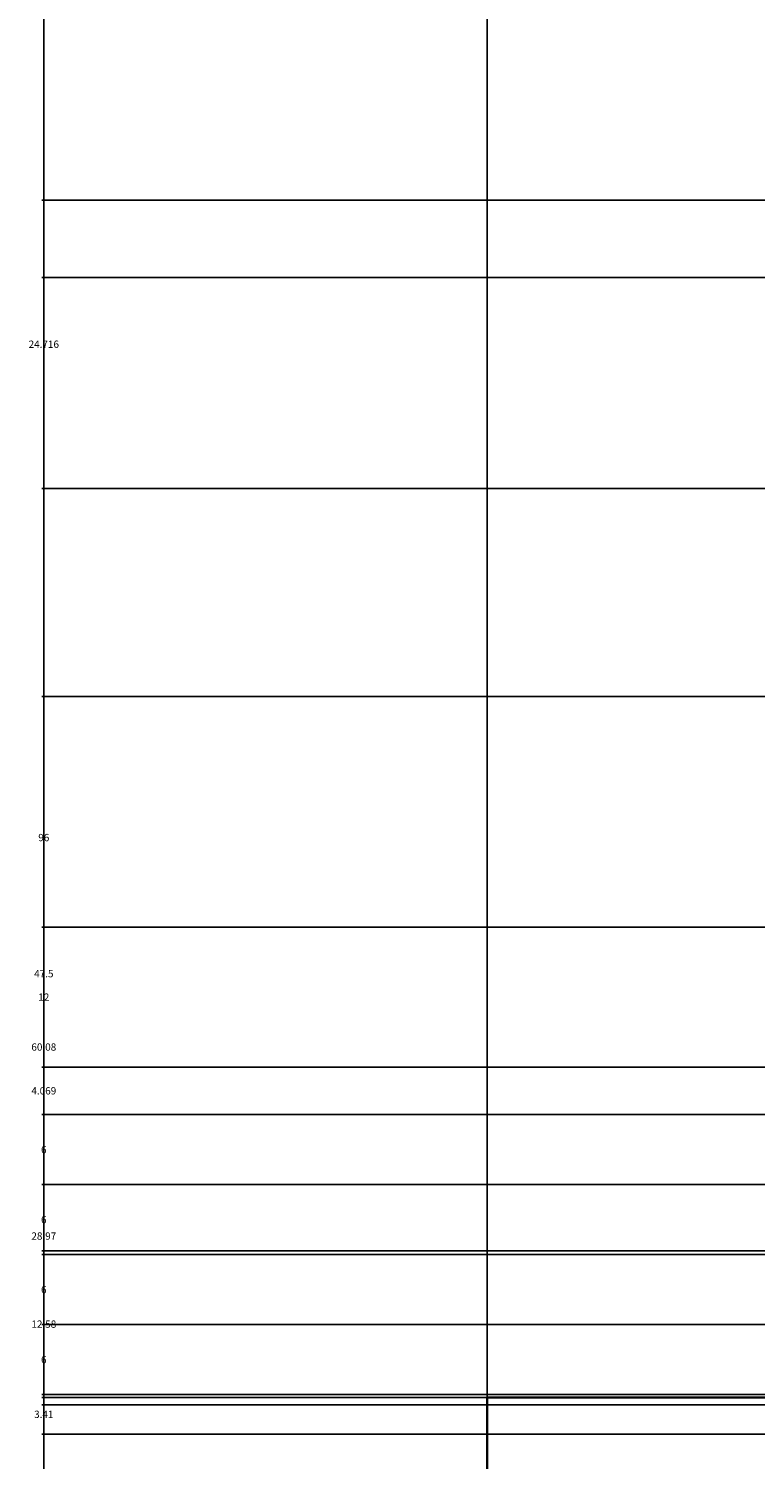
# Model space of a CAD drawing. Units: inches. Extents: x -13 to 809, y 112 to 656.
# Tile 3 of 55: x -13 to 49, y 205 to 328. Entities that reach past the tile are written whole.
import ezdxf

# ---------------------------------------------------------------- set-up
doc = ezdxf.new("R2010")
doc.units = ezdxf.units.IN
doc.header["$MEASUREMENT"] = 0
doc.layers.add('A-ANNO-DIMS', color=2, linetype='Continuous', lineweight=18)
doc.layers.add('A-ELEV', color=7, linetype='Continuous', lineweight=35)
doc.styles.get("Standard").update_dxf_attribs({"font": 'arial.ttf'})
doc.dimstyles.get("Standard").update_dxf_attribs({"dimtxt": 0.625, "dimasz": 0.18, "dimexe": 0.18, "dimexo": 0.0625, "dimgap": 0.09, "dimtad": 0, "dimtih": 1, "dimtoh": 1, "dimdec": 4, "dimzin": 0, "dimdsep": 46, "dimlunit": 4, "dimtxsty": 'Standard', "dimcen": 0.09, "dimadec": 0, "dimazin": 0, "dimtfac": 1, "dimtdec": 4, "dimtofl": 0, "dimtmove": 0, "dimatfit": 3, "dimfxl": 1, "dimtolj": 1, "dimtzin": 0, "dimarcsym": 0})

# ---------------------------------------------------------------- blocks, each defined once
blk = doc.blocks.new('*D11')
at = {"layer": 'A-ANNO-DIMS', "color": 0, "lineweight": -2, "transparency": 16777216}
for p, q in [((95.05, 306.46), (95.05, 112.34)), ((26.08, 150.46), (26.08, 112.34)), ((26.26, 112.52), (59.42, 112.52)), ((94.87, 112.52), (61.71, 112.52))]:
    blk.add_line(p, q, dxfattribs=at)
at = {"layer": 'A-ANNO-DIMS', "color": 0, "transparency": 16777216}
for points in [[(26.26, 112.55), (26.26, 112.49), (26.08, 112.52)], [(94.87, 112.55), (94.87, 112.49), (95.05, 112.52)]]:
    blk.add_solid(points, dxfattribs=at)
at = {"layer": 'Defpoints', "color": 0, "transparency": 16777216}
for p in [(95.05, 306.52), (26.08, 150.52), (95.05, 112.52)]:
    blk.add_point(p, dxfattribs=at)
at = {"layer": 'A-ANNO-DIMS', "color": 0, "transparency": 16777216, "insert": (60.56, 112.52), "char_height": 0.625, "attachment_point": 5}
blk.add_mtext('\\A1;68.97', dxfattribs=at)
blk = doc.blocks.new('*D22')
at = {"layer": 'A-ANNO-DIMS', "color": 0, "lineweight": -2, "transparency": 16777216}
for p, q in [((26.08, 210.58), (26.08, 655.96)), ((26.26, 655.78), (65.52, 655.78)), ((107.08, 655.78), (67.82, 655.78)), ((107.26, 510.58), (107.26, 655.96))]:
    blk.add_line(p, q, dxfattribs=at)
at = {"layer": 'A-ANNO-DIMS', "color": 0, "transparency": 16777216}
for points in [[(26.26, 655.81), (26.26, 655.75), (26.08, 655.78)], [(107.08, 655.81), (107.08, 655.75), (107.26, 655.78)]]:
    blk.add_solid(points, dxfattribs=at)
at = {"layer": 'Defpoints', "color": 0, "transparency": 16777216}
for p in [(107.26, 655.78), (107.26, 510.52), (26.08, 210.52)]:
    blk.add_point(p, dxfattribs=at)
at = {"layer": 'A-ANNO-DIMS', "color": 0, "transparency": 16777216, "insert": (66.67, 655.78), "char_height": 0.625, "attachment_point": 5}
blk.add_mtext('\\A1;81.18', dxfattribs=at)
blk = doc.blocks.new('*D32')
at = {"layer": 'A-ANNO-DIMS', "color": 0, "lineweight": -2, "transparency": 16777216}
for p, q in [((26.02, 210.52), (-12.1, 210.52)), ((-11.92, 210.34), (-11.92, 180.93)), ((-11.92, 150.7), (-11.92, 180.11)), ((26.02, 150.52), (-12.1, 150.52))]:
    blk.add_line(p, q, dxfattribs=at)
at = {"layer": 'A-ANNO-DIMS', "color": 0, "transparency": 16777216}
for points in [[(-11.95, 210.34), (-11.89, 210.34), (-11.92, 210.52)], [(-11.95, 150.7), (-11.89, 150.7), (-11.92, 150.52)]]:
    blk.add_solid(points, dxfattribs=at)
at = {"layer": 'Defpoints', "color": 0, "transparency": 16777216}
for p in [(-11.92, 210.52), (26.08, 210.52), (26.08, 150.52)]:
    blk.add_point(p, dxfattribs=at)
at = {"layer": 'A-ANNO-DIMS', "color": 0, "transparency": 16777216, "insert": (-11.92, 180.52), "char_height": 0.625, "attachment_point": 5}
blk.add_mtext('\\A1;60', dxfattribs=at)
blk = doc.blocks.new('*D33')
at = {"layer": 'A-ANNO-DIMS', "color": 0, "lineweight": -2, "transparency": 16777216}
for p, q in [((94.98, 306.52), (-12.1, 306.52)), ((-11.92, 306.34), (-11.92, 258.93)), ((-11.92, 210.7), (-11.92, 258.11)), ((26.02, 210.52), (-12.1, 210.52))]:
    blk.add_line(p, q, dxfattribs=at)
at = {"layer": 'A-ANNO-DIMS', "color": 0, "transparency": 16777216}
for points in [[(-11.95, 306.34), (-11.89, 306.34), (-11.92, 306.52)], [(-11.95, 210.7), (-11.89, 210.7), (-11.92, 210.52)]]:
    blk.add_solid(points, dxfattribs=at)
at = {"layer": 'Defpoints', "color": 0, "transparency": 16777216}
for p in [(-11.92, 306.52), (95.05, 306.52), (26.08, 210.52)]:
    blk.add_point(p, dxfattribs=at)
at = {"layer": 'A-ANNO-DIMS', "color": 0, "transparency": 16777216, "insert": (-11.92, 258.52), "char_height": 0.625, "attachment_point": 5}
blk.add_mtext('\\A1;96', dxfattribs=at)
blk = doc.blocks.new('*D34')
at = {"layer": 'A-ANNO-DIMS', "color": 0, "lineweight": -2, "transparency": 16777216}
for p, q in [((94.98, 462.52), (-12.1, 462.52)), ((-11.92, 462.34), (-11.92, 384.93)), ((-11.92, 306.7), (-11.92, 384.11)), ((94.98, 306.52), (-12.1, 306.52))]:
    blk.add_line(p, q, dxfattribs=at)
at = {"layer": 'A-ANNO-DIMS', "color": 0, "transparency": 16777216}
for points in [[(-11.95, 462.34), (-11.89, 462.34), (-11.92, 462.52)], [(-11.95, 306.7), (-11.89, 306.7), (-11.92, 306.52)]]:
    blk.add_solid(points, dxfattribs=at)
at = {"layer": 'Defpoints', "color": 0, "transparency": 16777216}
for p in [(-11.92, 462.52), (95.05, 462.52), (95.05, 306.52)]:
    blk.add_point(p, dxfattribs=at)
at = {"layer": 'A-ANNO-DIMS', "color": 0, "transparency": 16777216, "insert": (-11.92, 384.52), "char_height": 0.625, "attachment_point": 5}
blk.add_mtext('\\A1;156', dxfattribs=at)
blk = doc.blocks.new('*D39')
at = {"layer": 'A-ANNO-DIMS', "color": 0, "lineweight": -2, "transparency": 16777216}
for p, q in [((341.34, 524.28), (-12.1, 524.28)), ((-11.92, 524.1), (-11.92, 406.78)), ((-11.92, 288.63), (-11.92, 405.96)), ((341.34, 288.45), (-12.1, 288.45))]:
    blk.add_line(p, q, dxfattribs=at)
at = {"layer": 'A-ANNO-DIMS', "color": 0, "transparency": 16777216}
for points in [[(-11.95, 524.1), (-11.89, 524.1), (-11.92, 524.28)], [(-11.95, 288.63), (-11.89, 288.63), (-11.92, 288.45)]]:
    blk.add_solid(points, dxfattribs=at)
at = {"layer": 'Defpoints', "color": 0, "transparency": 16777216}
for p in [(-11.92, 524.28), (341.41, 524.28), (341.41, 288.45)]:
    blk.add_point(p, dxfattribs=at)
at = {"layer": 'A-ANNO-DIMS', "color": 0, "transparency": 16777216, "insert": (-11.92, 406.37), "char_height": 0.625, "attachment_point": 5}
blk.add_mtext('\\A1;235.83', dxfattribs=at)
blk = doc.blocks.new('*D40')
at = {"layer": 'A-ANNO-DIMS', "color": 0, "lineweight": -2, "transparency": 16777216}
for p, q in [((471.04, 313.17), (-12.1, 313.17)), ((-11.92, 312.99), (-11.92, 301.22)), ((-11.92, 288.63), (-11.92, 300.4)), ((341.34, 288.45), (-12.1, 288.45))]:
    blk.add_line(p, q, dxfattribs=at)
at = {"layer": 'A-ANNO-DIMS', "color": 0, "transparency": 16777216}
for points in [[(-11.95, 312.99), (-11.89, 312.99), (-11.92, 313.17)], [(-11.95, 288.63), (-11.89, 288.63), (-11.92, 288.45)]]:
    blk.add_solid(points, dxfattribs=at)
at = {"layer": 'Defpoints', "color": 0, "transparency": 16777216}
for p in [(471.1, 313.17), (-11.92, 288.45), (341.41, 288.45)]:
    blk.add_point(p, dxfattribs=at)
at = {"layer": 'A-ANNO-DIMS', "color": 0, "transparency": 16777216, "insert": (-11.92, 300.81), "char_height": 0.625, "attachment_point": 5}
blk.add_mtext('\\A1;24.716', dxfattribs=at)
blk = doc.blocks.new('*D41')
at = {"layer": 'A-ANNO-DIMS', "color": 0, "lineweight": -2, "transparency": 16777216}
for p, q in [((471.04, 357.98), (-12.1, 357.98)), ((-11.92, 357.8), (-11.92, 335.98)), ((-11.92, 313.35), (-11.92, 335.16)), ((471.04, 313.17), (-12.1, 313.17))]:
    blk.add_line(p, q, dxfattribs=at)
at = {"layer": 'A-ANNO-DIMS', "color": 0, "transparency": 16777216}
for points in [[(-11.95, 357.8), (-11.89, 357.8), (-11.92, 357.98)], [(-11.95, 313.35), (-11.89, 313.35), (-11.92, 313.17)]]:
    blk.add_solid(points, dxfattribs=at)
at = {"layer": 'Defpoints', "color": 0, "transparency": 16777216}
for p in [(-11.92, 357.98), (471.1, 357.98), (471.1, 313.17)]:
    blk.add_point(p, dxfattribs=at)
at = {"layer": 'A-ANNO-DIMS', "color": 0, "transparency": 16777216, "insert": (-11.92, 335.57), "char_height": 0.625, "attachment_point": 5}
blk.add_mtext('\\A1;44.81', dxfattribs=at)
blk = doc.blocks.new('*D44')
at = {"layer": 'A-ANNO-DIMS', "color": 0, "lineweight": -2, "transparency": 16777216}
for p, q in [((124.86, 270.6), (-12.1, 270.6)), ((-11.92, 270.42), (-11.92, 240.97)), ((-11.92, 210.7), (-11.92, 240.15)), ((124.86, 210.52), (-12.1, 210.52))]:
    blk.add_line(p, q, dxfattribs=at)
at = {"layer": 'A-ANNO-DIMS', "color": 0, "transparency": 16777216}
for points in [[(-11.95, 270.42), (-11.89, 270.42), (-11.92, 270.6)], [(-11.95, 210.7), (-11.89, 210.7), (-11.92, 210.52)]]:
    blk.add_solid(points, dxfattribs=at)
at = {"layer": 'Defpoints', "color": 0, "transparency": 16777216}
for p in [(-11.92, 270.6), (124.92, 270.6), (124.92, 210.52)]:
    blk.add_point(p, dxfattribs=at)
at = {"layer": 'A-ANNO-DIMS', "color": 0, "transparency": 16777216, "insert": (-11.92, 240.56), "char_height": 0.625, "attachment_point": 5}
blk.add_mtext('\\A1;60.08', dxfattribs=at)
blk = doc.blocks.new('*D45')
at = {"layer": 'A-ANNO-DIMS', "color": 0, "lineweight": -2, "transparency": 16777216}
for p, q in [((275.65, 270.6), (-12.1, 270.6)), ((-11.92, 270.42), (-11.92, 247.26)), ((-11.92, 223.28), (-11.92, 246.44)), ((275.65, 223.1), (-12.1, 223.1))]:
    blk.add_line(p, q, dxfattribs=at)
at = {"layer": 'A-ANNO-DIMS', "color": 0, "transparency": 16777216}
for points in [[(-11.95, 270.42), (-11.89, 270.42), (-11.92, 270.6)], [(-11.95, 223.28), (-11.89, 223.28), (-11.92, 223.1)]]:
    blk.add_solid(points, dxfattribs=at)
at = {"layer": 'Defpoints', "color": 0, "transparency": 16777216}
for p in [(-11.92, 270.6), (275.71, 270.6), (275.71, 223.1)]:
    blk.add_point(p, dxfattribs=at)
at = {"layer": 'A-ANNO-DIMS', "color": 0, "transparency": 16777216, "insert": (-11.92, 246.85), "char_height": 0.625, "attachment_point": 5}
blk.add_mtext('\\A1;47.5', dxfattribs=at)
blk = doc.blocks.new('*D49')
at = {"layer": 'A-ANNO-DIMS', "color": 0, "lineweight": -2, "transparency": 16777216}
for p, q in [((590.95, 250.84), (-12.1, 250.84)), ((-11.92, 250.66), (-11.92, 245.25)), ((-11.92, 239.02), (-11.92, 244.44)), ((590.95, 238.84), (-12.1, 238.84))]:
    blk.add_line(p, q, dxfattribs=at)
at = {"layer": 'A-ANNO-DIMS', "color": 0, "transparency": 16777216}
for points in [[(-11.95, 250.66), (-11.89, 250.66), (-11.92, 250.84)], [(-11.95, 239.02), (-11.89, 239.02), (-11.92, 238.84)]]:
    blk.add_solid(points, dxfattribs=at)
at = {"layer": 'Defpoints', "color": 0, "transparency": 16777216}
for p in [(-11.92, 250.84), (591.01, 250.84), (591.01, 238.84)]:
    blk.add_point(p, dxfattribs=at)
at = {"layer": 'A-ANNO-DIMS', "color": 0, "transparency": 16777216, "insert": (-11.92, 244.84), "char_height": 0.625, "attachment_point": 5}
blk.add_mtext('\\A1;12', dxfattribs=at)
blk = doc.blocks.new('*D50')
at = {"layer": 'A-ANNO-DIMS', "color": 0, "lineweight": -2, "transparency": 16777216}
for p, q in [((590.95, 238.84), (-12.1, 238.84)), ((-11.92, 238.66), (-11.92, 224.77)), ((-11.92, 210.06), (-11.92, 223.95)), ((607.51, 209.88), (-12.1, 209.88))]:
    blk.add_line(p, q, dxfattribs=at)
at = {"layer": 'A-ANNO-DIMS', "color": 0, "transparency": 16777216}
for points in [[(-11.95, 238.66), (-11.89, 238.66), (-11.92, 238.84)], [(-11.95, 210.06), (-11.89, 210.06), (-11.92, 209.88)]]:
    blk.add_solid(points, dxfattribs=at)
at = {"layer": 'Defpoints', "color": 0, "transparency": 16777216}
for p in [(591.01, 238.84), (-11.92, 209.88), (607.57, 209.88)]:
    blk.add_point(p, dxfattribs=at)
at = {"layer": 'A-ANNO-DIMS', "color": 0, "transparency": 16777216, "insert": (-11.92, 224.36), "char_height": 0.625, "attachment_point": 5}
blk.add_mtext('\\A1;28.97', dxfattribs=at)
blk = doc.blocks.new('*D80')
at = {"layer": 'A-ANNO-DIMS', "color": 0, "lineweight": -2, "transparency": 16777216}
for p, q in [((368.83, 216.77), (-12.1, 216.77)), ((-11.92, 216.59), (-11.92, 214.18)), ((-11.92, 210.95), (-11.92, 213.36)), ((368.83, 210.77), (-12.1, 210.77))]:
    blk.add_line(p, q, dxfattribs=at)
at = {"layer": 'A-ANNO-DIMS', "color": 0, "transparency": 16777216}
for points in [[(-11.95, 216.59), (-11.89, 216.59), (-11.92, 216.77)], [(-11.95, 210.95), (-11.89, 210.95), (-11.92, 210.77)]]:
    blk.add_solid(points, dxfattribs=at)
at = {"layer": 'Defpoints', "color": 0, "transparency": 16777216}
for p in [(-11.92, 216.77), (368.9, 216.77), (368.9, 210.77)]:
    blk.add_point(p, dxfattribs=at)
at = {"layer": 'A-ANNO-DIMS', "color": 0, "transparency": 16777216, "insert": (-11.92, 213.77), "char_height": 0.625, "attachment_point": 5}
blk.add_mtext('\\A1;6', dxfattribs=at)
blk = doc.blocks.new('*D81')
at = {"layer": 'A-ANNO-DIMS', "color": 0, "lineweight": -2, "transparency": 16777216}
for p, q in [((378.83, 222.77), (-12.1, 222.77)), ((-11.92, 222.59), (-11.92, 220.18)), ((-11.92, 216.95), (-11.92, 219.36)), ((378.83, 216.77), (-12.1, 216.77))]:
    blk.add_line(p, q, dxfattribs=at)
at = {"layer": 'A-ANNO-DIMS', "color": 0, "transparency": 16777216}
for points in [[(-11.95, 222.59), (-11.89, 222.59), (-11.92, 222.77)], [(-11.95, 216.95), (-11.89, 216.95), (-11.92, 216.77)]]:
    blk.add_solid(points, dxfattribs=at)
at = {"layer": 'Defpoints', "color": 0, "transparency": 16777216}
for p in [(-11.92, 222.77), (378.9, 222.77), (378.9, 216.77)]:
    blk.add_point(p, dxfattribs=at)
at = {"layer": 'A-ANNO-DIMS', "color": 0, "transparency": 16777216, "insert": (-11.92, 219.77), "char_height": 0.625, "attachment_point": 5}
blk.add_mtext('\\A1;6', dxfattribs=at)
blk = doc.blocks.new('*D82')
at = {"layer": 'A-ANNO-DIMS', "color": 0, "lineweight": -2, "transparency": 16777216}
for p, q in [((388.83, 228.77), (-12.1, 228.77)), ((-11.92, 228.59), (-11.92, 226.18)), ((-11.92, 222.95), (-11.92, 225.36)), ((388.83, 222.77), (-12.1, 222.77))]:
    blk.add_line(p, q, dxfattribs=at)
at = {"layer": 'A-ANNO-DIMS', "color": 0, "transparency": 16777216}
for points in [[(-11.95, 228.59), (-11.89, 228.59), (-11.92, 228.77)], [(-11.95, 222.95), (-11.89, 222.95), (-11.92, 222.77)]]:
    blk.add_solid(points, dxfattribs=at)
at = {"layer": 'Defpoints', "color": 0, "transparency": 16777216}
for p in [(-11.92, 228.77), (388.9, 228.77), (388.9, 222.77)]:
    blk.add_point(p, dxfattribs=at)
at = {"layer": 'A-ANNO-DIMS', "color": 0, "transparency": 16777216, "insert": (-11.92, 225.77), "char_height": 0.625, "attachment_point": 5}
blk.add_mtext('\\A1;6', dxfattribs=at)
blk = doc.blocks.new('*D83')
at = {"layer": 'A-ANNO-DIMS', "color": 0, "lineweight": -2, "transparency": 16777216}
for p, q in [((398.83, 234.77), (-12.1, 234.77)), ((-11.92, 234.59), (-11.92, 232.18)), ((-11.92, 228.95), (-11.92, 231.36)), ((398.83, 228.77), (-12.1, 228.77))]:
    blk.add_line(p, q, dxfattribs=at)
at = {"layer": 'A-ANNO-DIMS', "color": 0, "transparency": 16777216}
for points in [[(-11.95, 234.59), (-11.89, 234.59), (-11.92, 234.77)], [(-11.95, 228.95), (-11.89, 228.95), (-11.92, 228.77)]]:
    blk.add_solid(points, dxfattribs=at)
at = {"layer": 'Defpoints', "color": 0, "transparency": 16777216}
for p in [(-11.92, 234.77), (398.9, 234.77), (398.9, 228.77)]:
    blk.add_point(p, dxfattribs=at)
at = {"layer": 'A-ANNO-DIMS', "color": 0, "transparency": 16777216, "insert": (-11.92, 231.77), "char_height": 0.625, "attachment_point": 5}
blk.add_mtext('\\A1;6', dxfattribs=at)
blk = doc.blocks.new('*D84')
at = {"layer": 'A-ANNO-DIMS', "color": 0, "lineweight": -2, "transparency": 16777216}
for p, q in [((408.83, 238.84), (-12.1, 238.84)), ((-11.92, 238.66), (-11.92, 237.22)), ((-11.92, 234.95), (-11.92, 236.4)), ((408.83, 234.77), (-12.1, 234.77))]:
    blk.add_line(p, q, dxfattribs=at)
at = {"layer": 'A-ANNO-DIMS', "color": 0, "transparency": 16777216}
for points in [[(-11.95, 238.66), (-11.89, 238.66), (-11.92, 238.84)], [(-11.95, 234.95), (-11.89, 234.95), (-11.92, 234.77)]]:
    blk.add_solid(points, dxfattribs=at)
at = {"layer": 'Defpoints', "color": 0, "transparency": 16777216}
for p in [(-11.92, 238.84), (408.9, 238.84), (408.9, 234.77)]:
    blk.add_point(p, dxfattribs=at)
at = {"layer": 'A-ANNO-DIMS', "color": 0, "transparency": 16777216, "insert": (-11.92, 236.81), "char_height": 0.625, "attachment_point": 5}
blk.add_mtext('\\A1;4.069', dxfattribs=at)
blk = doc.blocks.new('*D90')
at = {"layer": 'A-ANNO-DIMS', "color": 0, "lineweight": -2, "transparency": 16777216}
for p, q in [((26.08, 210.46), (26.08, 112.34)), ((76.47, 195.83), (76.47, 112.34)), ((26.26, 112.52), (50.13, 112.52)), ((76.29, 112.52), (52.42, 112.52))]:
    blk.add_line(p, q, dxfattribs=at)
at = {"layer": 'A-ANNO-DIMS', "color": 0, "transparency": 16777216}
for points in [[(26.26, 112.55), (26.26, 112.49), (26.08, 112.52)], [(76.29, 112.55), (76.29, 112.49), (76.47, 112.52)]]:
    blk.add_solid(points, dxfattribs=at)
at = {"layer": 'Defpoints', "color": 0, "transparency": 16777216}
for p in [(26.08, 210.52), (76.47, 195.89), (76.47, 112.52)]:
    blk.add_point(p, dxfattribs=at)
at = {"layer": 'A-ANNO-DIMS', "color": 0, "transparency": 16777216, "insert": (51.28, 112.52), "char_height": 0.625, "attachment_point": 5}
blk.add_mtext('\\A1;50.39', dxfattribs=at)
blk = doc.blocks.new('*D94')
at = {"layer": 'A-ANNO-DIMS', "color": 0, "lineweight": -2, "transparency": 16777216}
for p, q in [((210.02, 223.1), (-12.1, 223.1)), ((-11.92, 222.92), (-11.92, 217.22)), ((-11.92, 210.7), (-11.92, 216.4)), ((160.86, 210.52), (-12.1, 210.52))]:
    blk.add_line(p, q, dxfattribs=at)
at = {"layer": 'A-ANNO-DIMS', "color": 0, "transparency": 16777216}
for points in [[(-11.95, 222.92), (-11.89, 222.92), (-11.92, 223.1)], [(-11.95, 210.7), (-11.89, 210.7), (-11.92, 210.52)]]:
    blk.add_solid(points, dxfattribs=at)
at = {"layer": 'Defpoints', "color": 0, "transparency": 16777216}
for p in [(-11.92, 223.1), (210.08, 223.1), (160.92, 210.52)]:
    blk.add_point(p, dxfattribs=at)
at = {"layer": 'A-ANNO-DIMS', "color": 0, "transparency": 16777216, "insert": (-11.92, 216.81), "char_height": 0.625, "attachment_point": 5}
blk.add_mtext('\\A1;12.58', dxfattribs=at)
blk = doc.blocks.new('*D115')
at = {"layer": 'A-ANNO-DIMS', "color": 0, "lineweight": -2, "transparency": 16777216}
for p, q in [((311.4, 210.78), (-12.1, 210.78)), ((-11.92, 210.6), (-11.92, 181.06)), ((-11.92, 150.7), (-11.92, 180.24)), ((311.64, 150.52), (-12.1, 150.52))]:
    blk.add_line(p, q, dxfattribs=at)
at = {"layer": 'A-ANNO-DIMS', "color": 0, "transparency": 16777216}
for points in [[(-11.95, 210.6), (-11.89, 210.6), (-11.92, 210.78)], [(-11.95, 150.7), (-11.89, 150.7), (-11.92, 150.52)]]:
    blk.add_solid(points, dxfattribs=at)
at = {"layer": 'Defpoints', "color": 0, "transparency": 16777216}
for p in [(-11.92, 210.78), (311.46, 210.78), (311.7, 150.52)]:
    blk.add_point(p, dxfattribs=at)
at = {"layer": 'A-ANNO-DIMS', "color": 0, "transparency": 16777216, "insert": (-11.92, 180.65), "char_height": 0.625, "attachment_point": 5}
blk.add_mtext('\\A1;60.27', dxfattribs=at)
blk = doc.blocks.new('*D118')
at = {"layer": 'A-ANNO-DIMS', "color": 0, "lineweight": -2, "transparency": 16777216}
for p, q in [((311.4, 210.78), (-12.1, 210.78)), ((-11.92, 210.6), (-11.92, 209.49)), ((-11.92, 207.55), (-11.92, 208.67)), ((308.59, 207.37), (-12.1, 207.37))]:
    blk.add_line(p, q, dxfattribs=at)
at = {"layer": 'A-ANNO-DIMS', "color": 0, "transparency": 16777216}
for points in [[(-11.95, 210.6), (-11.89, 210.6), (-11.92, 210.78)], [(-11.95, 207.55), (-11.89, 207.55), (-11.92, 207.37)]]:
    blk.add_solid(points, dxfattribs=at)
at = {"layer": 'Defpoints', "color": 0, "transparency": 16777216}
for p in [(-11.92, 210.78), (311.46, 210.78), (308.65, 207.37)]:
    blk.add_point(p, dxfattribs=at)
at = {"layer": 'A-ANNO-DIMS', "color": 0, "transparency": 16777216, "insert": (-11.92, 209.08), "char_height": 0.625, "attachment_point": 5}
blk.add_mtext('\\A1;3.41', dxfattribs=at)

msp = doc.modelspace()

# ---------------------------------------------------------------- linework, layer by layer
at = {"layer": 'A-ELEV'}
for q in [(256.4464, 210.5199), (26.0809, 150.5199)]:
    msp.add_line((26.0809, 210.5199), q, dxfattribs=at)

# ---------------------------------------------------------------- dimensions: what is measured, and where the dimension line sits
at = {"layer": 'A-ANNO-DIMS'}
for base, p1, p2, picture, middle in [((107.2588, 655.7828), (26.0809, 210.5199), (107.2588, 510.5199), '*D22', (66.6698, 655.7828)), ((95.0469, 112.5199), (26.0809, 150.5199), (95.0469, 306.5199), '*D11', (60.5639, 112.5199)), ((76.4733, 112.5199), (26.0809, 210.5199), (76.4733, 195.8907), '*D90', (51.2771, 112.5199))]:
    dim = msp.add_linear_dim(base=base, p1=p1, p2=p2, dimstyle='Standard', override={"dimdec": 2, "dimlfac": 1, "dimrnd": 0, "dimzin": 0, "dimdsep": 46, "dimlunit": 2}, dxfattribs=at)
    dim.commit()
    dim.dimension.update_dxf_attribs({"geometry": picture, "text_midpoint": middle})
for base, p1, p2, override, picture, middle in [((-11.9191, 524.281), (341.4072, 288.4508), (341.4072, 524.281), {"dimdec": 2, "dimlfac": 1, "dimrnd": 0, "dimzin": 0, "dimdsep": 46, "dimlunit": 2}, '*D39', (-11.9191, 406.3659)), ((-11.9191, 462.5199), (95.0469, 306.5199), (95.0469, 462.5199), {"dimdec": 0, "dimlfac": 1, "dimrnd": 0, "dimzin": 0, "dimdsep": 46, "dimlunit": 2}, '*D34', (-11.9191, 384.5199)), ((-11.9191, 357.9804), (471.0998, 313.1667), (471.0998, 357.9804), {"dimdec": 2, "dimlfac": 1, "dimrnd": 0, "dimzin": 0, "dimdsep": 46, "dimlunit": 2}, '*D41', (-11.9191, 335.5735)), ((-11.9191, 288.4508), (471.0998, 313.1667), (341.4072, 288.4508), {"dimdec": 3, "dimlfac": 1, "dimrnd": 0, "dimzin": 0, "dimdsep": 46, "dimlunit": 2}, '*D40', (-11.9191, 300.8087)), ((-11.9191, 306.5199), (26.0809, 210.5199), (95.0469, 306.5199), {"dimdec": 0, "dimlfac": 1, "dimrnd": 0, "dimzin": 0, "dimdsep": 46, "dimlunit": 2}, '*D33', (-11.9191, 258.5199)), ((-11.9191, 270.6024), (124.9184, 210.5199), (124.9184, 270.6024), {"dimdec": 2, "dimlfac": 1, "dimrnd": 0, "dimzin": 0, "dimdsep": 46, "dimlunit": 2}, '*D44', (-11.9191, 240.5611)), ((-11.9191, 270.6024), (275.7145, 223.1), (275.7145, 270.6024), {"dimdec": 1, "dimlfac": 1, "dimrnd": 0, "dimzin": 0, "dimdsep": 46, "dimlunit": 2}, '*D45', (-11.9191, 246.8512)), ((-11.9191, 250.8429), (591.008, 238.8429), (591.008, 250.8429), {"dimdec": 0, "dimlfac": 1, "dimrnd": 0, "dimzin": 0, "dimdsep": 46, "dimlunit": 2}, '*D49', (-11.9191, 244.8429)), ((-11.9191, 209.8753), (591.008, 238.8429), (607.5741, 209.8753), {"dimdec": 2, "dimlfac": 1, "dimrnd": 0, "dimzin": 0, "dimdsep": 46, "dimlunit": 2}, '*D50', (-11.9191, 224.3591)), ((-11.9191, 238.8429), (408.8966, 234.7738), (408.8966, 238.8429), {"dimdec": 3, "dimlfac": 1, "dimrnd": 0, "dimzin": 0, "dimdsep": 46, "dimlunit": 2}, '*D84', (-11.9191, 236.8083)), ((-11.9191, 234.7738), (398.8966, 228.7738), (398.8966, 234.7738), {"dimdec": 0, "dimlfac": 1, "dimrnd": 0, "dimzin": 0, "dimdsep": 46, "dimlunit": 2}, '*D83', (-11.9191, 231.7738)), ((-11.9191, 228.7738), (388.8966, 222.7738), (388.8966, 228.7738), {"dimdec": 0, "dimlfac": 1, "dimrnd": 0, "dimzin": 0, "dimdsep": 46, "dimlunit": 2}, '*D82', (-11.9191, 225.7738)), ((-11.9191, 223.1), (160.9184, 210.5199), (210.0791, 223.1), {"dimdec": 2, "dimlfac": 1, "dimrnd": 0, "dimzin": 0, "dimdsep": 46, "dimlunit": 2}, '*D94', (-11.9191, 216.81)), ((-11.9191, 222.7738), (378.8966, 216.7738), (378.8966, 222.7738), {"dimdec": 0, "dimlfac": 1, "dimrnd": 0, "dimzin": 0, "dimdsep": 46, "dimlunit": 2}, '*D81', (-11.9191, 219.7738)), ((-11.9191, 216.7738), (368.8966, 210.7738), (368.8966, 216.7738), {"dimdec": 0, "dimlfac": 1, "dimrnd": 0, "dimzin": 0, "dimdsep": 46, "dimlunit": 2}, '*D80', (-11.9191, 213.7738)), ((-11.91915, 210.78493), (311.6991, 150.51989), (311.46269, 210.78493), {"dimdec": 2, "dimlfac": 1, "dimrnd": 0, "dimzin": 0, "dimdsep": 46, "dimlunit": 2}, '*D115', (-11.91915, 180.65241)), ((-11.9191, 210.7849), (308.6488, 207.3724), (311.4627, 210.7849), {"dimdec": 2, "dimlfac": 1, "dimrnd": 0, "dimzin": 0, "dimdsep": 46, "dimlunit": 2}, '*D118', (-11.9191, 209.0787)), ((-11.9191, 210.5199), (26.0809, 150.5199), (26.0809, 210.5199), {"dimdec": 0, "dimlfac": 1, "dimrnd": 0, "dimzin": 0, "dimdsep": 46, "dimlunit": 2}, '*D32', (-11.9191, 180.5199))]:
    dim = msp.add_linear_dim(base=base, p1=p1, p2=p2, angle=90, dimstyle='Standard', override=override, dxfattribs=at)
    dim.commit()
    dim.dimension.update_dxf_attribs({"geometry": picture, "text_midpoint": middle})

doc.saveas('drawing.dxf')
